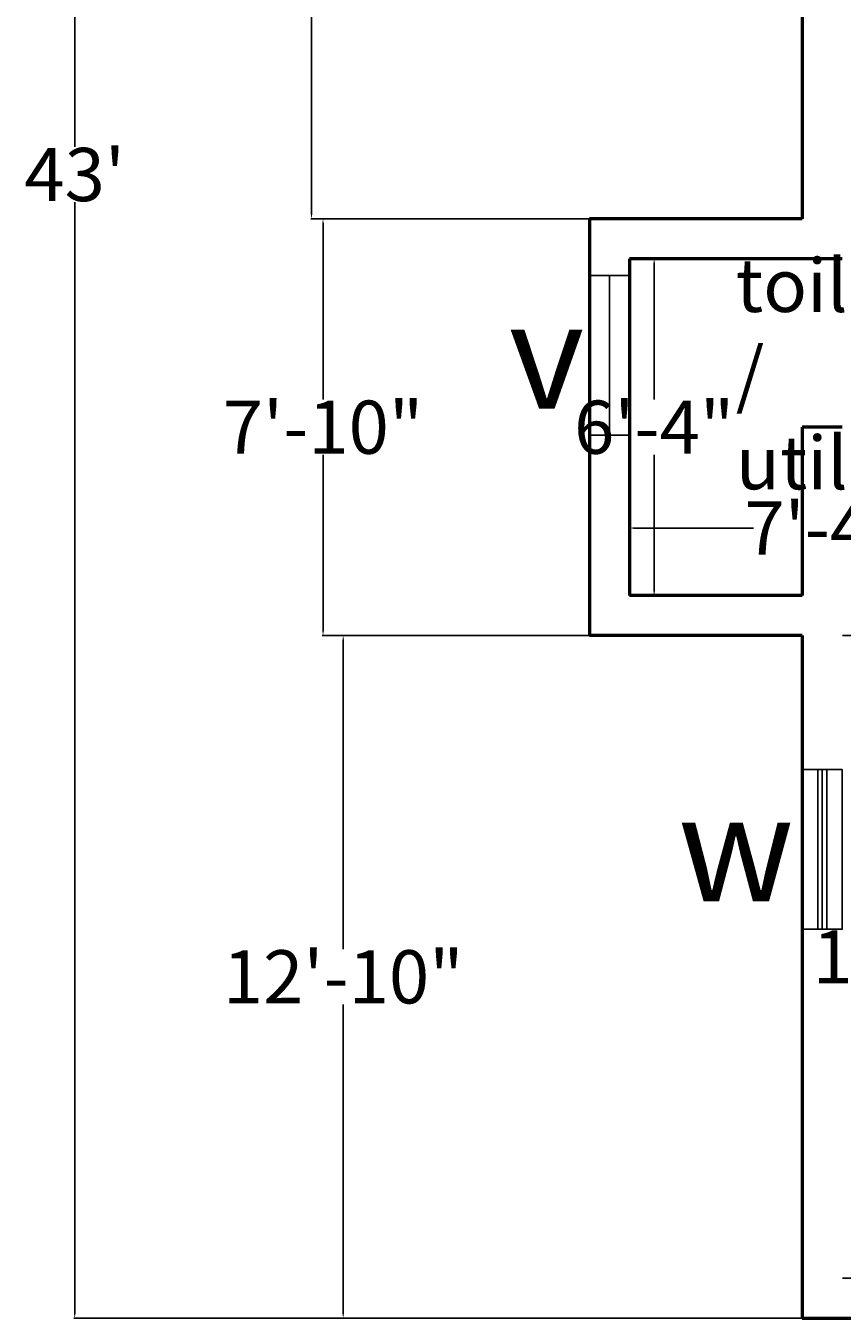
# Model space of a CAD drawing. Units: inches. Extents: x 409 to 7572, y 7 to 725.
# Tile 14 of 38: x 2800 to 2984, y 157 to 448. Entities that reach past the tile are written whole.
import ezdxf

# ---------------------------------------------------------------- set-up
doc = ezdxf.new("R2010")
doc.units = ezdxf.units.IN
doc.header["$MEASUREMENT"] = 0
for name, color, linetype, lineweight in [('A-ANNO-DIMS', 2, 'Continuous', 18), ('A-ANNO-SYMB', 3, 'Continuous', 25), ('A-AREA-IDEN', 7, 'Continuous', 25), ('A-GLAZ', 4, 'Continuous', 25), ('A-WALL', 7, 'Continuous', 50)]:
    doc.layers.add(name, color=color, linetype=linetype, lineweight=lineweight)
doc.styles.get("Standard").update_dxf_attribs({"font": 'arial.ttf'})
doc.dimstyles.get("Standard").update_dxf_attribs({"dimtxt": 2, "dimasz": 1, "dimexe": 0.18, "dimexo": 0.0625, "dimgap": 0.09, "dimtad": 0, "dimtih": 1, "dimtoh": 1, "dimdec": 0, "dimzin": 0, "dimdsep": 46, "dimlunit": 3, "dimtxsty": 'Standard', "dimcen": 0.09, "dimadec": 0, "dimazin": 0, "dimtfac": 1, "dimtdec": 0, "dimtofl": 0, "dimtmove": 0, "dimatfit": 3, "dimfxl": 1, "dimtolj": 1, "dimtzin": 0, "dimarcsym": 0})

# ---------------------------------------------------------------- blocks, each defined once
blk = doc.blocks.new('*D70')
at = {"layer": 'A-ANNO-DIMS', "color": 0, "lineweight": -2, "transparency": 16777216}
for p, q in [((2984.16, 310.53), (3000.2, 310.53)), ((3000.02, 309.53), (3000.02, 244.15)), ((3000.02, 166.53), (3000.02, 231.92)), ((2984.16, 165.53), (3000.2, 165.53))]:
    blk.add_line(p, q, dxfattribs=at)
at = {"layer": 'A-ANNO-DIMS', "color": 0, "transparency": 16777216}
for points in [[(2999.85, 309.53), (3000.19, 309.53), (3000.02, 310.53)], [(2999.85, 166.53), (3000.19, 166.53), (3000.02, 165.53)]]:
    blk.add_solid(points, dxfattribs=at)
at = {"layer": 'DEFPOINTS', "color": 0, "transparency": 16777216}
for p in [(2984.1, 310.53), (2984.1, 165.53), (3000.02, 165.53)]:
    blk.add_point(p, dxfattribs=at)
at = {"layer": 'A-ANNO-DIMS', "color": 0, "transparency": 16777216, "insert": (3000.02, 238.03), "char_height": 2, "attachment_point": 5}
blk.add_mtext('\\A1;{\\H6x;12\'-1"}', dxfattribs=at)
blk = doc.blocks.new('*D87')
at = {"layer": 'A-ANNO-DIMS', "color": 0, "lineweight": -2, "transparency": 16777216}
for p, q in [((2945.3, 395.53), (2941.48, 395.53)), ((2941.66, 394.53), (2941.66, 363.75)), ((2941.66, 320.53), (2941.66, 351.31)), ((2945.3, 319.53), (2941.48, 319.53))]:
    blk.add_line(p, q, dxfattribs=at)
at = {"layer": 'A-ANNO-DIMS', "color": 0, "transparency": 16777216}
for points in [[(2941.49, 394.53), (2941.83, 394.53), (2941.66, 395.53)], [(2941.49, 320.53), (2941.83, 320.53), (2941.66, 319.53)]]:
    blk.add_solid(points, dxfattribs=at)
at = {"layer": 'DEFPOINTS', "color": 0, "transparency": 16777216}
for p in [(2945.36, 395.53), (2941.66, 319.53), (2945.36, 319.53)]:
    blk.add_point(p, dxfattribs=at)
at = {"layer": 'A-ANNO-DIMS', "color": 0, "transparency": 16777216, "insert": (2941.66, 357.53), "char_height": 2, "attachment_point": 5}
blk.add_mtext('\\A1;{\\H6x;6\'-4"}', dxfattribs=at)
blk = doc.blocks.new('*D89')
at = {"layer": 'A-ANNO-DIMS', "color": 0, "lineweight": -2, "transparency": 16777216}
for p, q in [((2936.1, 346.33), (2936.1, 334.6)), ((3024.1, 346.33), (3024.1, 334.6)), ((2937.1, 334.78), (2964.11, 334.78)), ((3023.1, 334.78), (2996.09, 334.78))]:
    blk.add_line(p, q, dxfattribs=at)
at = {"layer": 'A-ANNO-DIMS', "color": 0, "transparency": 16777216}
for points in [[(2937.1, 334.95), (2937.1, 334.61), (2936.1, 334.78)], [(3023.1, 334.95), (3023.1, 334.61), (3024.1, 334.78)]]:
    blk.add_solid(points, dxfattribs=at)
at = {"layer": 'DEFPOINTS', "color": 0, "transparency": 16777216}
for p in [(2936.1, 346.39), (3024.1, 346.39), (3024.1, 334.78)]:
    blk.add_point(p, dxfattribs=at)
at = {"layer": 'A-ANNO-DIMS', "color": 0, "transparency": 16777216, "insert": (2980.1, 334.78), "char_height": 2, "attachment_point": 5}
blk.add_mtext('\\A1;{\\H6x;7\'-4"}', dxfattribs=at)
blk = doc.blocks.new('*D76')
at = {"layer": 'A-ANNO-DIMS', "color": 0, "lineweight": -2, "transparency": 16777216}
for p, q in [((2975.04, 672.53), (2864.14, 672.53)), ((2864.32, 671.53), (2864.32, 544.65)), ((2864.32, 405.53), (2864.32, 532.42)), ((2975.04, 404.53), (2864.14, 404.53))]:
    blk.add_line(p, q, dxfattribs=at)
at = {"layer": 'A-ANNO-DIMS', "color": 0, "transparency": 16777216}
for points in [[(2864.15, 671.53), (2864.48, 671.53), (2864.32, 672.53)], [(2864.15, 405.53), (2864.48, 405.53), (2864.32, 404.53)]]:
    blk.add_solid(points, dxfattribs=at)
at = {"layer": 'DEFPOINTS', "color": 0, "transparency": 16777216}
for p in [(2975.1, 672.53), (2864.32, 404.53), (2975.1, 404.53)]:
    blk.add_point(p, dxfattribs=at)
at = {"layer": 'A-ANNO-DIMS', "color": 0, "transparency": 16777216, "insert": (2864.32, 538.53), "char_height": 2, "attachment_point": 5}
blk.add_mtext('\\A1;{\\H6x;22\'-4"}', dxfattribs=at)
blk = doc.blocks.new('*D77')
at = {"layer": 'A-ANNO-DIMS', "color": 0, "lineweight": -2, "transparency": 16777216}
for p, q in [((2927.04, 404.53), (2866.73, 404.53)), ((2866.91, 403.53), (2866.91, 363.75)), ((2866.91, 311.53), (2866.91, 351.31)), ((2927.04, 310.53), (2866.73, 310.53))]:
    blk.add_line(p, q, dxfattribs=at)
at = {"layer": 'A-ANNO-DIMS', "color": 0, "transparency": 16777216}
for points in [[(2866.74, 403.53), (2867.07, 403.53), (2866.91, 404.53)], [(2866.74, 311.53), (2867.07, 311.53), (2866.91, 310.53)]]:
    blk.add_solid(points, dxfattribs=at)
at = {"layer": 'DEFPOINTS', "color": 0, "transparency": 16777216}
for p in [(2927.1, 404.53), (2866.91, 310.53), (2927.1, 310.53)]:
    blk.add_point(p, dxfattribs=at)
at = {"layer": 'A-ANNO-DIMS', "color": 0, "transparency": 16777216, "insert": (2866.91, 357.53), "char_height": 2, "attachment_point": 5}
blk.add_mtext('\\A1;{\\H6x;7\'-10"}', dxfattribs=at)
blk = doc.blocks.new('*D78')
at = {"layer": 'A-ANNO-DIMS', "color": 0, "lineweight": -2, "transparency": 16777216}
for p, q in [((2975.04, 310.53), (2871.29, 310.53)), ((2871.47, 309.53), (2871.47, 239.75)), ((2871.47, 157.53), (2871.47, 227.31)), ((2975.04, 156.53), (2871.29, 156.53))]:
    blk.add_line(p, q, dxfattribs=at)
at = {"layer": 'A-ANNO-DIMS', "color": 0, "transparency": 16777216}
for points in [[(2871.3, 309.53), (2871.63, 309.53), (2871.47, 310.53)], [(2871.3, 157.53), (2871.63, 157.53), (2871.47, 156.53)]]:
    blk.add_solid(points, dxfattribs=at)
at = {"layer": 'DEFPOINTS', "color": 0, "transparency": 16777216}
for p in [(2975.1, 310.53), (2871.47, 156.53), (2975.1, 156.53)]:
    blk.add_point(p, dxfattribs=at)
at = {"layer": 'A-ANNO-DIMS', "color": 0, "transparency": 16777216, "insert": (2871.47, 233.53), "char_height": 2, "attachment_point": 5}
blk.add_mtext('\\A1;{\\H6x;12\'-10"}', dxfattribs=at)
blk = doc.blocks.new('*D65')
at = {"layer": 'A-ANNO-DIMS', "color": 0, "lineweight": -2, "transparency": 16777216}
for p, q in [((2975.04, 672.53), (2810.68, 672.53)), ((2810.86, 671.53), (2810.86, 420.75)), ((2810.86, 157.53), (2810.86, 408.31)), ((2975.04, 156.53), (2810.68, 156.53))]:
    blk.add_line(p, q, dxfattribs=at)
at = {"layer": 'A-ANNO-DIMS', "color": 0, "transparency": 16777216}
for points in [[(2810.69, 671.53), (2811.03, 671.53), (2810.86, 672.53)], [(2810.69, 157.53), (2811.03, 157.53), (2810.86, 156.53)]]:
    blk.add_solid(points, dxfattribs=at)
at = {"layer": 'DEFPOINTS', "color": 0, "transparency": 16777216}
for p in [(2975.1, 672.53), (2810.86, 156.53), (2975.1, 156.53)]:
    blk.add_point(p, dxfattribs=at)
at = {"layer": 'A-ANNO-DIMS', "color": 0, "transparency": 16777216, "insert": (2810.86, 414.53), "char_height": 2, "attachment_point": 5}
blk.add_mtext("\\A1;{\\H6x;43'}", dxfattribs=at)
blk = doc.blocks.new('WIN-36')
for p, q in [((1699.82, 514.65), (1699.82, 478.65)), ((1700.82, 514.65), (1700.82, 478.65)), ((1701.82, 514.65), (1701.82, 478.65))]:
    blk.add_line(p, q)
blk.add_lwpolyline([(1705.32, 514.65), (1705.32, 478.65), (1696.32, 478.65), (1696.32, 514.65)], close=True)
blk = doc.blocks.new('VENT-36')
blk.add_line((5633.28, 355.73), (5633.28, 391.73))
blk.add_lwpolyline([(5628.78, 355.73), (5628.78, 391.73), (5637.78, 391.73), (5637.78, 355.73)], close=True)

msp = doc.modelspace()

# ---------------------------------------------------------------- linework, layer by layer
at = {"layer": 'A-WALL'}
for p, q in [((2975.1, 672.53), (2975.1, 404.53)), ((2975.1, 404.53), (2927.1, 404.53)), ((2927.1, 404.53), (2927.1, 310.53)), ((2984.1, 395.53), (2936.1, 395.53)), ((2936.1, 395.53), (2936.1, 319.53)), ((2975.1, 357.53), (2975.1, 319.53)), ((2984.1, 357.53), (2975.1, 357.53)), ((2975.1, 319.53), (2936.1, 319.53)), ((2975.1, 310.53), (2927.1, 310.53)), ((2975.1, 310.53), (2975.1, 156.53)), ((2975.1, 156.53), (3349.1, 156.53))]:
    msp.add_line(p, q, dxfattribs=at)

# ---------------------------------------------------------------- block references
at = {"layer": 'A-GLAZ'}
for name, p in [('VENT-36', (-2701.69, 0)), ('WIN-36', (1278.78, -234.38))]:
    msp.add_blockref(name, p, dxfattribs=at)

# ---------------------------------------------------------------- texts
at = {"layer": 'A-ANNO-SYMB', "char_height": 24, "attachment_point": 1}
for s, insert in [('v', (2908.84, 385.73)), ('w', (2947, 274.54))]:
    msp.add_mtext_dynamic_manual_height_columns(s, width=18.2582, gutter_width=1, heights=[0], dxfattribs=dict(at, insert=insert))
at = {"layer": 'A-AREA-IDEN', "insert": (2960.1, 395.53), "char_height": 12, "attachment_point": 1}
msp.add_mtext_dynamic_manual_height_columns('toilet / utility', width=49.2946, gutter_width=1, heights=[0], dxfattribs=at)

# ---------------------------------------------------------------- dimensions: what is measured, and where the dimension line sits
at = {"layer": 'A-ANNO-DIMS'}
for base, p1, p2, picture, middle in [((2810.86, 156.53), (2975.1, 672.53), (2975.1, 156.53), '*D65', (2810.86, 414.53)), ((2864.32, 404.53), (2975.1, 672.53), (2975.1, 404.53), '*D76', (2864.32, 538.53)), ((2866.91, 310.53), (2927.1, 404.53), (2927.1, 310.53), '*D77', (2866.91, 357.53)), ((2941.66, 319.53), (2945.36, 395.53), (2945.36, 319.53), '*D87', (2941.66, 357.53)), ((2871.47, 156.53), (2975.1, 310.53), (2975.1, 156.53), '*D78', (2871.47, 233.53)), ((3000.02, 165.53), (2984.1, 310.53), (2984.1, 165.53), '*D70', (3000.02, 238.03))]:
    dim = msp.add_linear_dim(base=base, p1=p1, p2=p2, angle=90, text='{\\H6x;<>}', dimstyle='Standard', override={"dimclrd": 0, "dimclre": 0, "dimclrt": 0}, dxfattribs=at)
    dim.commit()
    dim.dimension.update_dxf_attribs({"geometry": picture, "text_midpoint": middle})
dim = msp.add_linear_dim(base=(3024.1, 334.78), p1=(2936.1, 346.39), p2=(3024.1, 346.39), text='{\\H6x;<>}', dimstyle='Standard', override={"dimclrd": 0, "dimclre": 0, "dimclrt": 0}, dxfattribs=at)
dim.commit()
dim.dimension.update_dxf_attribs({"geometry": '*D89', "text_midpoint": (2980.1, 334.78)})

doc.saveas('drawing.dxf')
